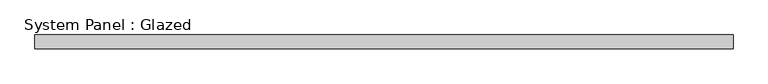
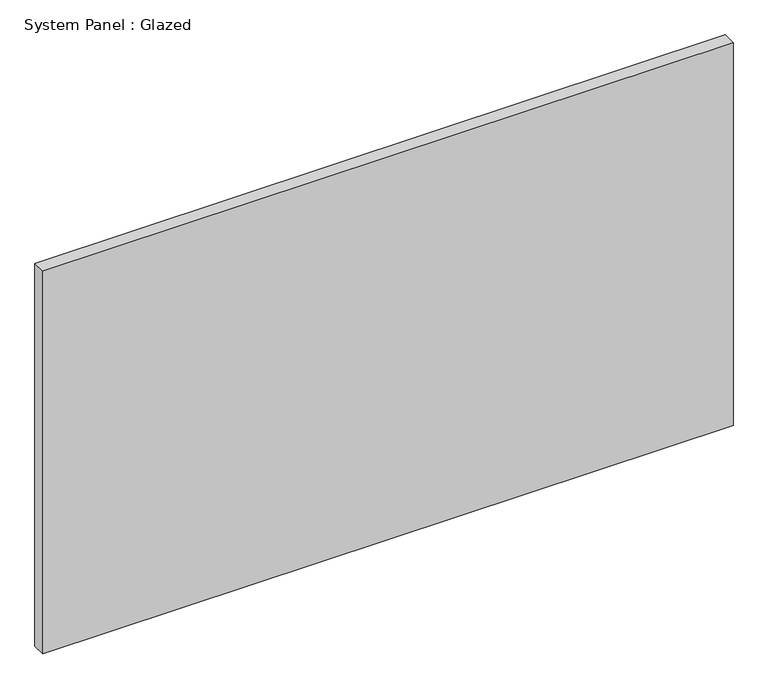
"""IFC4 building model written with IfcOpenShell, lengths in millimetres: plate geometry, System Panel : Glazed."""

from ifc_helpers import new_model, si_unit, origin, origin_with_axes, place, context, project, spatial, polyline, outline, extrude, source, transform, mapped, element, save


def system_panel_glazed_060269ed(model_context):
    return source(origin(), model_context, "Body", "SweptSolid", [
        extrude(outline(polyline([(645.5833333, 19.05), (-645.5833333, 19.05), (-645.5833333, 44.45), (645.5833333, 44.45), (645.5833333, 19.05)])), origin_with_axes(), (0.0, 0.0, 1.0), 757.5270145),
    ])


if __name__ == "__main__":
    model = new_model("IFC4")
    model_context = context("Model", 3, world=origin())
    ifc_project = project(units=[si_unit("LENGTHUNIT", "METRE", prefix="MILLI")], contexts=[model_context])
    site = spatial("IfcSite", under=ifc_project)
    building = spatial("IfcBuilding", under=site)
    placement = place(None, origin())
    system_panel_glazed_shape = system_panel_glazed_060269ed(model_context)
    element("IfcPlate", 1, ObjectType="System Panel : Glazed", at=placement, inside=building, context=model_context, shape_type="MappedRepresentation", body=[
        mapped(system_panel_glazed_shape, transform((0.0, 0.0, 0.0), x_axis=(1.0, 0.0, 0.0), y_axis=(0.0, 1.0, 0.0), z_axis=(0.0, 0.0, 1.0))),
    ])
    save(model, "model.ifc")

# Revit data of these elements
# Type "System Panel : Glazed"
#   Construction Type Id = "GSP4R"
#   Analytic Construction = "1/8 in Pilkington single glazing"
#   Visual Light Transmittance = 0.9
#   Solar Heat Gain Coefficient = 0.86
#   Heat Transfer Coefficient (U) = 1.18115 BTU/(h·ft²·°F)
#   Define Thermal Properties by = 1
# Element 1 (IfcPlate, "System Panel : Glazed")
#   Materials on its faces: "Glass"
# Materials
#   "Glass": class "Glass", colour RGB 0 128 192, transparency 0.75, Description = "Soda Lime Glass", Cost = 0
